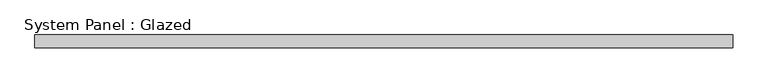
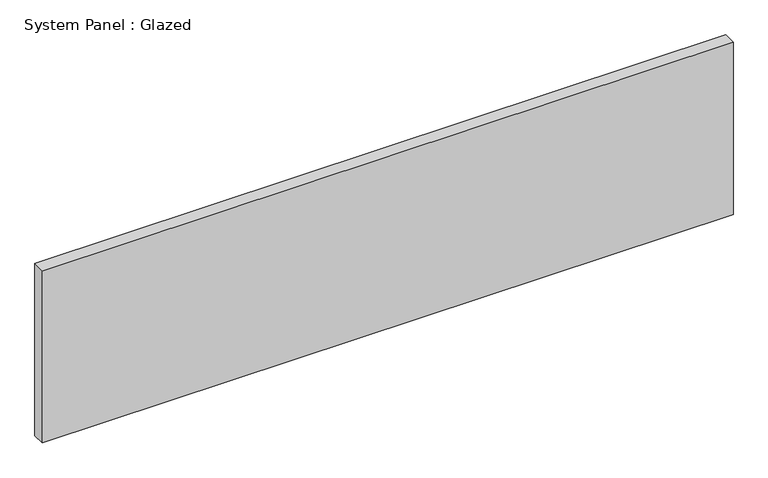
"""IFC4 building model written with IfcOpenShell, lengths in millimetres: plate geometry, System Panel : Glazed."""

from ifc_helpers import new_model, si_unit, origin, origin_with_axes, place, context, project, spatial, polyline, outline, extrude, source, transform, mapped, element, save


def system_panel_glazed_ee0060d4(model_context):
    return source(origin(), model_context, "Body", "SweptSolid", [
        extrude(outline(polyline([(685.7999999, 19.05), (-685.7999999, 19.05), (-685.7999999, 44.45), (685.7999999, 44.45), (685.7999999, 19.05)])), origin_with_axes(), (0.0, 0.0, 1.0), 361.95),
    ])


if __name__ == "__main__":
    model = new_model("IFC4")
    model_context = context("Model", 3, world=origin())
    ifc_project = project(units=[si_unit("LENGTHUNIT", "METRE", prefix="MILLI")], contexts=[model_context])
    site = spatial("IfcSite", under=ifc_project)
    building = spatial("IfcBuilding", under=site)
    placement = place(None, origin())
    system_panel_glazed_shape = system_panel_glazed_ee0060d4(model_context)
    element("IfcPlate", 1, ObjectType="System Panel : Glazed", at=placement, inside=building, context=model_context, shape_type="MappedRepresentation", body=[
        mapped(system_panel_glazed_shape, transform((0.0, 0.0, 0.0), x_axis=(1.0, 0.0, 0.0), y_axis=(0.0, 1.0, 0.0), z_axis=(0.0, 0.0, 1.0))),
    ])
    save(model, "model.ifc")

# Revit data of these elements
# Type "System Panel : Glazed"
#   Construction Type Id = "GSP4R"
#   Analytic Construction = "1/8 in Pilkington single glazing"
#   Visual Light Transmittance = 0.9
#   Solar Heat Gain Coefficient = 0.86
#   Heat Transfer Coefficient (U) = 1.18115 BTU/(h·ft²·°F)
#   Define Thermal Properties by = 1
# Element 1 (IfcPlate, "System Panel : Glazed")
#   Materials on its faces: "Glass"
# Materials
#   "Glass": class "Glass", colour RGB 0 128 192, transparency 0.75, Description = "Soda Lime Glass", Cost = 0
